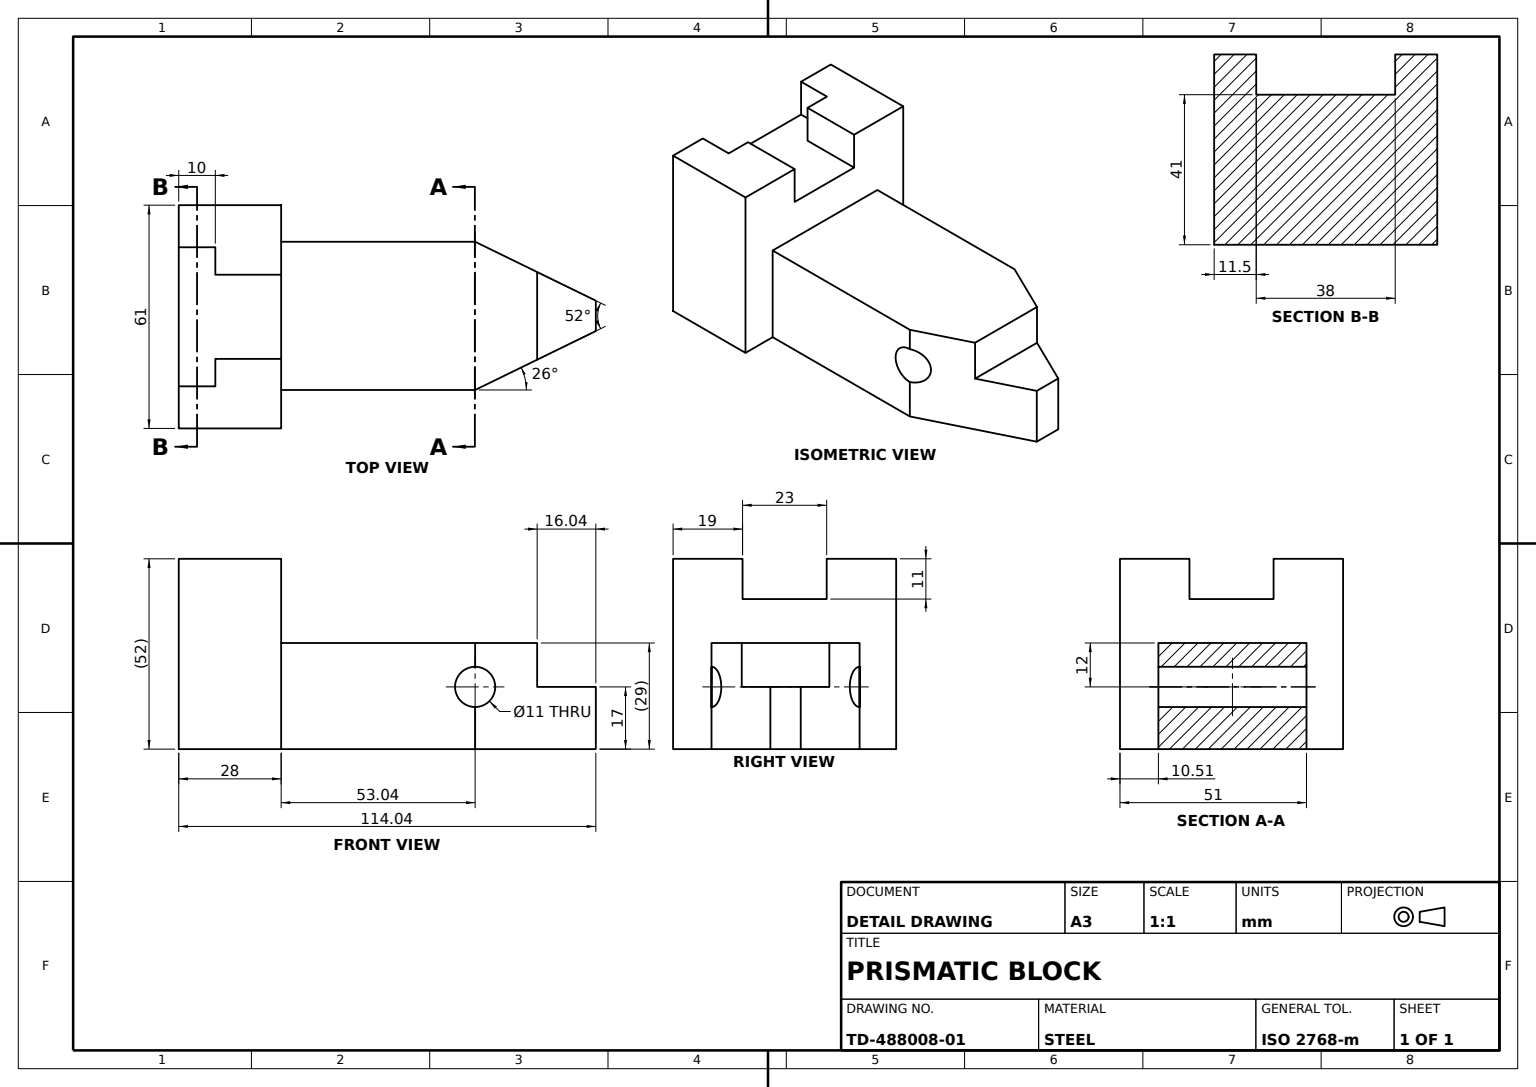
SolidWorks part; units mm, degrees
material "Plain Carbon Steel"
ref_plane "Front Plane" through (0, 0, 0) normal (0, 0, 1) x (1, 0, 0)
ref_plane "Top Plane" through (0, 0, 0) normal (0, 1, 0) x (1, 0, 0)
ref_plane "Right Plane" through (0, 0, 0) normal (1, 0, 0) x (0, 0, -1)
sketch "Base Block Profile" plane through (0, 0, 0) normal (0, 0, 1) x (1, 0, 0)
  line L1 (-30.5, 20.5) -> (30.5, 20.5)
  line L2 (-30.5, 20.5) -> (-30.5, -20.5)
  line L3 (-30.5, -20.5) -> (30.5, -20.5)
  line L4 (30.5, 20.5) -> (30.5, -20.5)
  line L5 (-30.5, 20.5) -> (30.5, -20.5) construction
  line L6 (-30.5, -20.5) -> (30.5, 20.5) construction
  point P0 (0, 0)
  dimension "D1" = 41
  dimension "D2" = 61
extrude "Base Block 41x61x120" add sketch "Base Block Profile" along normal blind 120
sketch "Step Cut Profile" plane through (30.5, 0, 0) normal (1, 0, 0) x (0, 0, -1)
  line L0 (0, -20.5) -> (0, -3.5)
  line L1 (0, -20.5) -> (0, 20.5) construction
  line L2 (0, -3.5) -> (-22, -3.5)
  line L3 (-22, -3.5) -> (-22, 8.5)
  line L4 (-22, 8.5) -> (-92, 8.5)
  line L5 (-92, 8.5) -> (-92, 20.5)
  line L6 (-120, 20.5) -> (0, 20.5) construction
  line L7 (-92, 20.5) -> (0, 20.5)
  line L8 (0, 20.5) -> (0, -3.5)
  line L9 (-120, -20.5) -> (0, -20.5) construction
  line L10 (-120, -20.5) -> (-120, 20.5) construction
  line M4 (0, -20.5) -> (0, 20.5)
  line M5 (0, 20.5) -> (-120, 20.5)
  dimension "D1" = 29
  dimension "D2" = 12
  dimension "D3" = 12
  dimension "D4" = 28
  dimension "D5" = 22
  dimension "D6" = 41
extrude "Lengthwise Step Cut" cut sketch "Step Cut Profile" against normal blind 120 contours L5 L4 L3 L2 M4 M5
sketch "End Boss Layout Sketch" plane through (0, 20.5, 0) normal (0, 1, 0) x (1, 0, 0)
  line L0 (30.5, -120) -> (-30.5, -120) construction
  line L1 (-19, -110) -> (-11.5, -110)
  line L2 (-19, -110) -> (-19, -120)
  line L3 (-19, -120) -> (19, -120)
  line L4 (19, -110) -> (19, -120)
  line L5 (-19, -110) -> (19, -120) construction
  line L6 (-19, -120) -> (19, -110) construction
  line L7 (-30.5, -120) -> (-30.5, -92) construction
  line L8 (-30.5, -92) -> (30.5, -92) construction
  line L10 (-11.5, -110) -> (-11.5, -92)
  line L11 (-11.5, -92) -> (11.5, -92)
  line L12 (11.5, -110) -> (11.5, -92)
  line L13 (-11.5, -110) -> (11.5, -92) construction
  line L14 (-11.5, -92) -> (11.5, -110) construction
  line L15 (11.5, -110) -> (19, -110)
  point P0 (0, -115)
  point P9 (0, -101)
  dimension "D1" = 10
  dimension "D2" = 30.5
  dimension "D3" = 23
  dimension "D4" = 38
sketch "End Boss Profile" plane through (0, 20.5, 0) normal (0, 1, 0) x (1, 0, 0)
  line L6 (0, -120) -> (0, -106.0551) construction
  line L7 (-19, -120) -> (19, -120) construction
  line L14 (-19, -120) -> (-30.5, -120)
  line L15 (-30.5, -120) -> (-30.5, -92)
  line L16 (-30.5, -92) -> (-11.5, -92)
  line L17 (-11.5, -92) -> (-11.5, -110)
  line L18 (-11.5, -110) -> (-19, -110)
  line L19 (-19, -110) -> (-19, -120)
  line L20 (11.5, -92) -> (30.5, -92)
  line L21 (30.5, -92) -> (30.5, -120)
  line L22 (30.5, -120) -> (19, -120)
  line L23 (19, -120) -> (19, -110)
  line L24 (19, -110) -> (11.5, -110)
  line L25 (11.5, -110) -> (11.5, -92)
extrude "Castellated End Bosses" add sketch "End Boss Profile" along normal blind 11
sketch "Tapered Nose Profile" plane through (0, 0, 0) normal (0, 1, 0) x (1, 0, 0)
  line L6 (0, -92) -> (0, 29.5627) construction
  line L7 (-4.4048, -5.9558) -> (-20.5, -38.9558)
  line L8 (3.8987, -5.9558) -> (19.9939, -38.9558)
  line L9 (-30.5, 0) -> (30.5, 0) construction
  line L10 (-20.5, -92) -> (19.9939, -92)
  line L11 (-20.5, -92) -> (-20.5, -5.9558)
  line L13 (19.9939, -92) -> (19.9939, -5.9558)
  line L14 (-20.5, -92) -> (20.5, 0) construction
  line L15 (-20.4845, 1.1287) -> (19.9939, -92) construction
  line L16 (-11.5, -92) -> (11.5, -92) construction
  line L17 (-20.5, -5.9558) -> (19.9939, -5.9558)
  line L19 (-20.5, -5.9558) -> (-30.5, -5.9558)
  line L20 (-20.5, -5.9558) -> (-20.5, -92)
  line L21 (-20.5, -92) -> (-30.5, -92)
  line L22 (-30.5, -5.9558) -> (-30.5, -92)
  line L23 (19.9939, -5.9558) -> (30.5, -5.9558)
  line L24 (19.9939, -5.9558) -> (19.9939, -92)
  line L25 (19.9939, -92) -> (30.5, -92)
  line L26 (30.5, -5.9558) -> (30.5, -92)
  point P0 (0, -46)
  dimension "D1" = 41
  dimension "D2" = 52
  dimension "D3" = 26
  dimension "D4" = 33
  dimension "D5" = 20.5
  dimension "D6" = 34.3987
  dimension "D7" = 53.0442
extrude "Tapered Nose Cut" cut sketch "Tapered Nose Profile" against normal blind 51 and the other way through all contours L19 L22 L21 L11 | L26 L23 L13 L25 | L17 L8 L13 | L17 L11 L7
sketch "Nose Slot Profile" plane through (0, -3.5, 0) normal (0, 1, 0) x (1, 0, 0)
  line L8 (-30.5, -5.9558) -> (-4.4048, -5.9558)
  line L9 (-4.4048, -5.9558) -> (-12.2301, -22)
  line L10 (-12.2301, -22) -> (11.724, -22)
  line L11 (11.724, -22) -> (3.8987, -5.9558)
  line L12 (3.8987, -5.9558) -> (30.5, -5.9558)
  line L13 (30.5, -5.9558) -> (30.5, 0)
  line L14 (30.5, 0) -> (-30.5, 0)
  line L15 (-30.5, 0) -> (-30.5, -5.9558)
  line L16 (-30.5, -5.9558) -> (3.8987, -5.9558)
  line L17 (-4.4048, -5.9558) -> (-12.2301, -22)
  line L18 (-12.2301, -22) -> (11.724, -22)
  line L19 (11.724, -22) -> (3.8987, -5.9558)
  line L20 (3.8987, -5.9558) -> (30.5, -5.9558)
  line L21 (30.5, -5.9558) -> (30.5, 0)
  line L22 (30.5, 0) -> (-30.5, 0)
  line L23 (-30.5, 0) -> (-30.5, -5.9558)
  dimension "D1" = 0
extrude "Nose Slot Cut" cut sketch "Nose Slot Profile" against normal blind 51 contours L20 L21 L22 L23 L16
sketch "Cross Hole Profile" plane through (0, 0, 0) normal (1, 0, 0) x (0, 0, -1)
  line L0 (-38.9558, 8.5) -> (-38.9558, -20.5) construction
  line L1 (-38.9558, 8.5) -> (-22, 8.5) construction
  circle A0 centre (-38.9558, -3.5) radius 5.5
  dimension "D2" = 11
  dimension "D1" = 12
extrude "Cross Hole" cut sketch "Cross Hole Profile" against normal through all both and the other way through all
